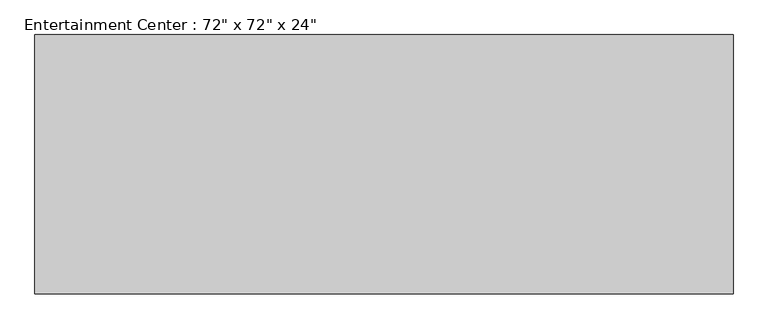
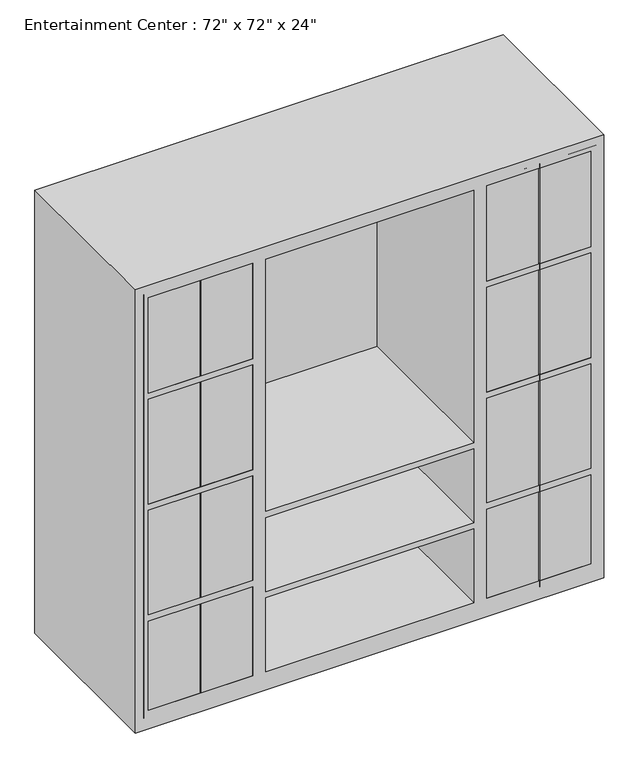
"""IFC4 building model written with IfcOpenShell, lengths in millimetres: furniture geometry."""

from ifc_helpers import new_model, si_unit, point, frame, frame_2d, origin, place, context, project, spatial, polyline, circle_curve, trimmed, segment, composite_curve, outline, extrude, faceted_brep, source, transform, mapped, element, save


def furniture_cf0b6580(model_context):
    return source(origin(), model_context, "Body", "SolidModel", [
        faceted_brep([(914.4, -781.05, 0.0), (914.4, -781.05, 1828.8), (-914.4, -781.05, 1828.8), (-914.4, -781.05, 0.0), (-457.2, -781.05, 1778.0), (-457.2, -781.05, 1384.3), (-863.6, -781.05, 1384.3), (-863.6, -781.05, 1778.0), (-457.2, -781.05, 76.2), (-863.6, -781.05, 76.2), (-863.6, -781.05, 444.5), (-457.2, -781.05, 444.5), (863.6, -781.05, 1384.3), (457.2, -781.05, 1384.3), (457.2, -781.05, 1778.0), (863.6, -781.05, 1778.0), (-406.4, -781.05, 736.6), (-406.4, -781.05, 1778.0), (406.4, -781.05, 1778.0), (406.4, -781.05, 736.6), (406.4, -781.05, 76.2), (-406.4, -781.05, 76.2), (-406.4, -781.05, 381.0), (406.4, -781.05, 381.0), (863.6, -781.05, 76.2), (457.2, -781.05, 76.2), (457.2, -781.05, 444.5), (863.6, -781.05, 444.5), (-863.6, -781.05, 469.9), (-863.6, -781.05, 901.7), (-457.2, -781.05, 901.7), (-457.2, -781.05, 469.9), (-457.2, -781.05, 1358.9), (-457.2, -781.05, 927.1), (-863.6, -781.05, 927.1), (-863.6, -781.05, 1358.9), (457.2, -781.05, 1358.9), (863.6, -781.05, 1358.9), (863.6, -781.05, 927.1), (457.2, -781.05, 927.1), (457.2, -781.05, 901.7), (863.6, -781.05, 901.7), (863.6, -781.05, 469.9), (457.2, -781.05, 469.9), (406.4, -781.05, 406.4), (-406.4, -781.05, 406.4), (-406.4, -781.05, 711.2), (406.4, -781.05, 711.2), (914.4, -101.6, 0.0), (-914.4, -101.6, 0.0), (-914.4, -101.6, 1828.8), (914.4, -101.6, 1828.8), (-457.2, -127.0, 1778.0), (-457.2, -127.0, 1384.3), (-863.6, -127.0, 1384.3), (-863.6, -127.0, 1778.0), (-457.2, -127.0, 76.2), (-863.6, -127.0, 76.2), (-863.6, -127.0, 444.5), (-457.2, -127.0, 444.5), (863.6, -127.0, 1384.3), (457.2, -127.0, 1384.3), (457.2, -127.0, 1778.0), (863.6, -127.0, 1778.0), (-406.4, -127.0, 736.6), (-406.4, -127.0, 1778.0), (406.4, -127.0, 1778.0), (406.4, -127.0, 736.6), (406.4, -127.0, 76.2), (-406.4, -127.0, 76.2), (-406.4, -127.0, 381.0), (406.4, -127.0, 381.0), (863.6, -127.0, 76.2), (457.2, -127.0, 76.2), (457.2, -127.0, 444.5), (863.6, -127.0, 444.5), (-863.6, -127.0, 469.9), (-863.6, -127.0, 901.7), (-457.2, -127.0, 901.7), (-457.2, -127.0, 469.9), (-457.2, -127.0, 1358.9), (-457.2, -127.0, 927.1), (-863.6, -127.0, 927.1), (-863.6, -127.0, 1358.9), (457.2, -127.0, 1358.9), (863.6, -127.0, 1358.9), (863.6, -127.0, 927.1), (457.2, -127.0, 927.1), (457.2, -127.0, 901.7), (863.6, -127.0, 901.7), (863.6, -127.0, 469.9), (457.2, -127.0, 469.9), (406.4, -127.0, 406.4), (-406.4, -127.0, 406.4), (-406.4, -127.0, 711.2), (406.4, -127.0, 711.2)], [[[0, 1, 2, 3], [4, 5, 6, 7], [8, 9, 10, 11], [12, 13, 14, 15], [16, 17, 18, 19], [20, 21, 22, 23], [24, 25, 26, 27], [28, 29, 30, 31], [32, 33, 34, 35], [36, 37, 38, 39], [40, 41, 42, 43], [44, 45, 46, 47]], [[48, 49, 50, 51]], [[1, 0, 48, 51]], [[2, 1, 51, 50]], [[3, 2, 50, 49]], [[0, 3, 49, 48]], [[5, 4, 52, 53]], [[6, 5, 53, 54]], [[7, 6, 54, 55]], [[4, 7, 55, 52]], [[9, 8, 56, 57]], [[10, 9, 57, 58]], [[11, 10, 58, 59]], [[8, 11, 59, 56]], [[13, 12, 60, 61]], [[14, 13, 61, 62]], [[15, 14, 62, 63]], [[12, 15, 63, 60]], [[17, 16, 64, 65]], [[18, 17, 65, 66]], [[19, 18, 66, 67]], [[16, 19, 67, 64]], [[21, 20, 68, 69]], [[22, 21, 69, 70]], [[23, 22, 70, 71]], [[20, 23, 71, 68]], [[25, 24, 72, 73]], [[26, 25, 73, 74]], [[27, 26, 74, 75]], [[24, 27, 75, 72]], [[29, 28, 76, 77]], [[30, 29, 77, 78]], [[31, 30, 78, 79]], [[28, 31, 79, 76]], [[33, 32, 80, 81]], [[34, 33, 81, 82]], [[35, 34, 82, 83]], [[32, 35, 83, 80]], [[37, 36, 84, 85]], [[38, 37, 85, 86]], [[39, 38, 86, 87]], [[36, 39, 87, 84]], [[41, 40, 88, 89]], [[42, 41, 89, 90]], [[43, 42, 90, 91]], [[40, 43, 91, 88]], [[45, 44, 92, 93]], [[46, 45, 93, 94]], [[47, 46, 94, 95]], [[44, 47, 95, 92]], [[53, 52, 55, 54]], [[57, 56, 59, 58]], [[61, 60, 63, 62]], [[65, 64, 67, 66]], [[69, 68, 71, 70]], [[73, 72, 75, 74]], [[77, 76, 79, 78]], [[81, 80, 83, 82]], [[85, 84, 87, 86]], [[89, 88, 91, 90]], [[93, 92, 95, 94]]]),
        extrude(outline(composite_curve([segment(polyline([(1003.3, -632.9986452), (1003.3, -657.225), (825.5, -657.225), (825.5, -632.9986452)]), True, "CONTINUOUS"), segment(trimmed(circle_curve(frame_2d((850.9, -632.9986452)), 25.4), [point((825.5, -632.9986452))], [point((850.9, -607.5986452))], False, "CARTESIAN"), True, "CONTINUOUS"), segment(polyline([(850.9, -607.5986452), (977.9, -607.5986452)]), True, "CONTINUOUS"), segment(trimmed(circle_curve(frame_2d((977.9, -632.9986452)), 25.4), [point((977.9, -607.5986452))], [point((1003.3, -632.9986452))], False, "CARTESIAN"), True, "CONTINUOUS")], self_intersect=False)), frame((0.0, -714.375, 0.0), z_axis=(0.0, 1.0, 0.0), x_axis=(0.0, 0.0, 1.0)), (0.0, 0.0, 1.0), 3.175),
        extrude(outline(composite_curve([segment(trimmed(circle_curve(frame_2d((977.9, -688.18125)), 25.4), [point((1003.3, -688.18125))], [point((977.9, -713.58125))], False, "CARTESIAN"), True, "CONTINUOUS"), segment(polyline([(977.9, -713.58125), (850.9, -713.58125)]), True, "CONTINUOUS"), segment(trimmed(circle_curve(frame_2d((850.9, -688.18125)), 25.4), [point((850.9, -713.58125))], [point((825.5, -688.18125))], False, "CARTESIAN"), True, "CONTINUOUS"), segment(polyline([(825.5, -688.18125), (825.5, -663.575), (1003.3, -663.575), (1003.3, -688.18125)]), True, "CONTINUOUS")], self_intersect=False)), frame((0.0, -714.375, 0.0), z_axis=(0.0, 1.0, 0.0), x_axis=(0.0, 0.0, 1.0)), (0.0, 0.0, 1.0), 3.175),
        extrude(outline(composite_curve([segment(trimmed(circle_curve(frame_2d((977.9, 632.9986452)), 25.4), [point((1003.3, 632.9986452))], [point((977.9, 607.5986452))], False, "CARTESIAN"), True, "CONTINUOUS"), segment(polyline([(977.9, 607.5986452), (850.9, 607.5986452)]), True, "CONTINUOUS"), segment(trimmed(circle_curve(frame_2d((850.9, 632.9986452)), 25.4), [point((850.9, 607.5986452))], [point((825.5, 632.9986452))], False, "CARTESIAN"), True, "CONTINUOUS"), segment(polyline([(825.5, 632.9986452), (825.5, 657.225), (1003.3, 657.225), (1003.3, 632.9986452)]), True, "CONTINUOUS")], self_intersect=False)), frame((0.0, -714.375, 0.0), z_axis=(0.0, 1.0, 0.0), x_axis=(0.0, 0.0, 1.0)), (0.0, 0.0, 1.0), 3.175),
        extrude(outline(composite_curve([segment(polyline([(1003.3, 688.18125), (1003.3, 663.575), (825.5, 663.575), (825.5, 688.18125)]), True, "CONTINUOUS"), segment(trimmed(circle_curve(frame_2d((850.9, 688.18125)), 25.4), [point((825.5, 688.18125))], [point((850.9, 713.58125))], False, "CARTESIAN"), True, "CONTINUOUS"), segment(polyline([(850.9, 713.58125), (977.9, 713.58125)]), True, "CONTINUOUS"), segment(trimmed(circle_curve(frame_2d((977.9, 688.18125)), 25.4), [point((977.9, 713.58125))], [point((1003.3, 688.18125))], False, "CARTESIAN"), True, "CONTINUOUS")], self_intersect=False)), frame((0.0, -714.375, 0.0), z_axis=(0.0, 1.0, 0.0), x_axis=(0.0, 0.0, 1.0)), (0.0, 0.0, 1.0), 3.175),
        extrude(outline(polyline([(-882.65, -711.2), (-663.575, -711.2), (-663.575, -781.05), (-882.65, -781.05), (-882.65, -711.2)])), frame((0.0, 0.0, 50.8), z_axis=(0.0, 0.0, 1.0), x_axis=(1.0, 0.0, 0.0)), (0.0, 0.0, 1.0), 1746.25),
        extrude(outline(polyline([(-657.225, -711.2), (-438.15, -711.2), (-438.15, -781.05), (-657.225, -781.05), (-657.225, -711.2)])), frame((0.0, 0.0, 50.8), z_axis=(0.0, 0.0, 1.0), x_axis=(1.0, 0.0, 0.0)), (0.0, 0.0, 1.0), 1746.25),
        extrude(outline(polyline([(663.575, -711.2), (882.65, -711.2), (882.65, -781.05), (663.575, -781.05), (663.575, -711.2)])), frame((0.0, 0.0, 50.8), z_axis=(0.0, 0.0, 1.0), x_axis=(1.0, 0.0, 0.0)), (0.0, 0.0, 1.0), 1746.25),
        extrude(outline(polyline([(438.15, -711.2), (657.225, -711.2), (657.225, -781.05), (438.15, -781.05), (438.15, -711.2)])), frame((0.0, 0.0, 50.8), z_axis=(0.0, 0.0, 1.0), x_axis=(1.0, 0.0, 0.0)), (0.0, 0.0, 1.0), 1746.25),
    ])


if __name__ == "__main__":
    model = new_model("IFC4")
    model_context = context("Model", 3, world=origin())
    ifc_project = project(units=[si_unit("LENGTHUNIT", "METRE", prefix="MILLI")], contexts=[model_context])
    site = spatial("IfcSite", under=ifc_project)
    building = spatial("IfcBuilding", under=site)
    placement = place(None, origin())
    furniture_shape = furniture_cf0b6580(model_context)
    element("IfcFurniture", 1, ObjectType="Entertainment Center : 72\" x 72\" x 24\"", at=placement, inside=building, context=model_context, shape_type="MappedRepresentation", body=[
        mapped(furniture_shape, transform((0.0, 0.0, 0.0), x_axis=(1.0, 0.0, 0.0), y_axis=(0.0, 1.0, 0.0), z_axis=(0.0, 0.0, 1.0))),
    ])
    save(model, "model.ifc")

# Revit data of these elements
# Type "Entertainment Center : 72\" x 72\" x 24\""
#   Assembly Code = "E2020200"
#   Center Width = 2' - 8"
#   Depth = 2' - 0"
#   Height = 6' - 0"
#   Width = 6' - 0"
#   Material = none
# Element 1 (IfcFurniture, "Entertainment Center : 72\" x 72\" x 24\"")
#   Materials on its faces: "Steel, Chrome Plated", "Glass - Clear, Grey"
# Materials
#   "Steel, Chrome Plated": class "Metal", colour RGB 17 17 17, transparency 0, Description = "Chromiuim plated steel", Cost = 0
#   "Glass - Clear, Grey": class "Glass", colour RGB 252 255 255, transparency 0.64
